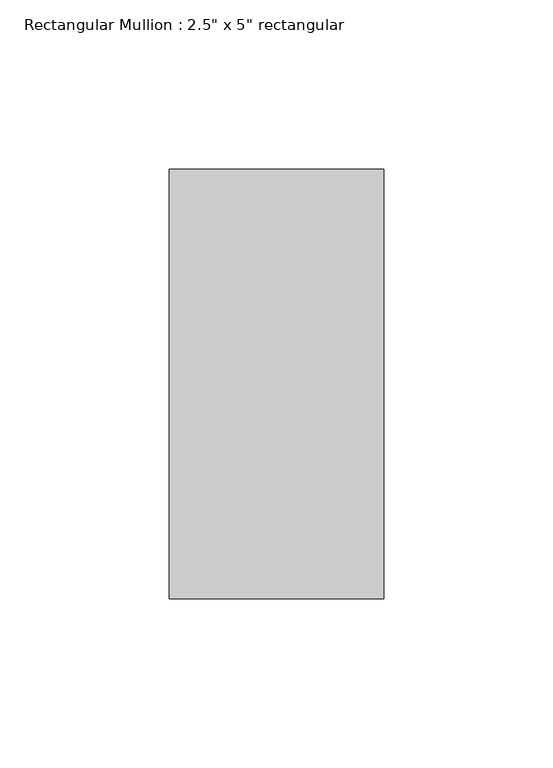
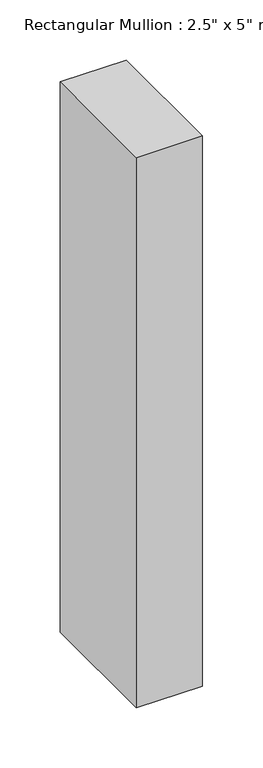
"""IFC4 building model written with IfcOpenShell, lengths in millimetres: member geometry."""

from ifc_helpers import new_model, si_unit, frame, origin, place, context, project, spatial, polyline, outline, extrude, source, transform, mapped, element, save


def member_bc554fa6(model_context):
    return source(origin(), model_context, "Body", "SweptSolid", [
        extrude(outline(polyline([(31.75, 63.5), (31.75, -63.5), (-31.75, -63.5), (-31.75, 63.5), (31.75, 63.5)])), frame((0.0, 0.0, -558.8), z_axis=(0.0, 0.0, 1.0), x_axis=(1.0, 0.0, 0.0)), (0.0, 0.0, 1.0), 558.8),
    ])


if __name__ == "__main__":
    model = new_model("IFC4")
    model_context = context("Model", 3, world=origin())
    ifc_project = project(units=[si_unit("LENGTHUNIT", "METRE", prefix="MILLI")], contexts=[model_context])
    site = spatial("IfcSite", under=ifc_project)
    building = spatial("IfcBuilding", under=site)
    placement = place(None, origin())
    member_shape = member_bc554fa6(model_context)
    element("IfcMember", 1, ObjectType="Rectangular Mullion : 2.5\" x 5\" rectangular", at=placement, inside=building, context=model_context, shape_type="MappedRepresentation", body=[
        mapped(member_shape, transform((0.0, 0.0, 0.0), x_axis=(1.0, 0.0, 0.0), y_axis=(0.0, 1.0, 0.0), z_axis=(0.0, 0.0, 1.0))),
    ])
    save(model, "model.ifc")

# Revit data of these elements
# Type "Rectangular Mullion : 2.5\" x 5\" rectangular"
#   built-in parameter 1007304 = 0.416667 (stored number, unit not read)
#   built-in parameter 1007301 = 0.104167 (stored number, unit not read)
#   built-in parameter 1007300 = 0.104167 (stored number, unit not read)
# Element 1 (IfcMember, "Rectangular Mullion : 2.5\" x 5\" rectangular")
#   Materials on its faces: "Rectangle 1 sq"
# Materials
#   "Rectangle 1 sq": class "Generic", colour RGB 120 120 120, transparency 0, Cost = 0
